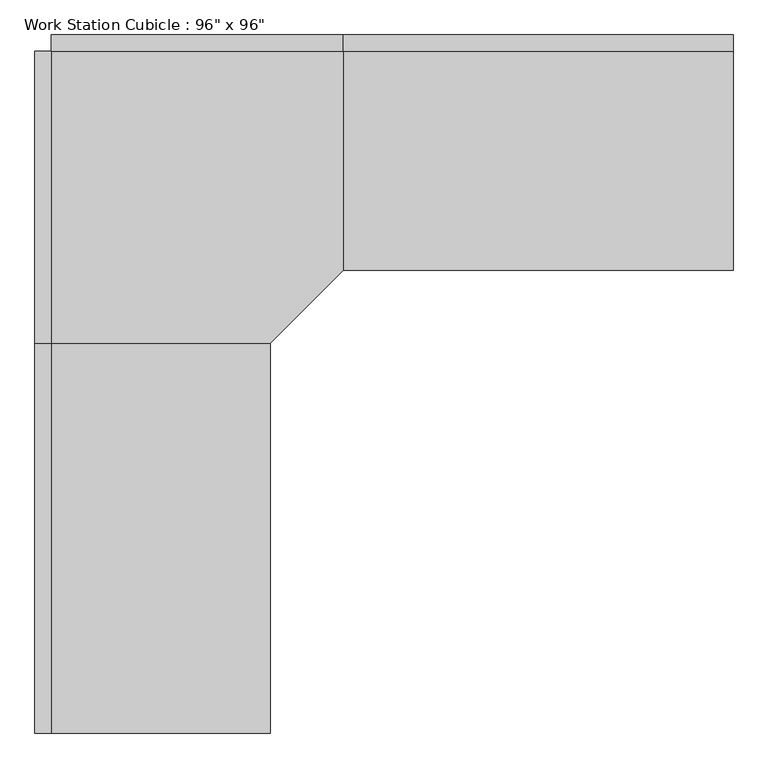
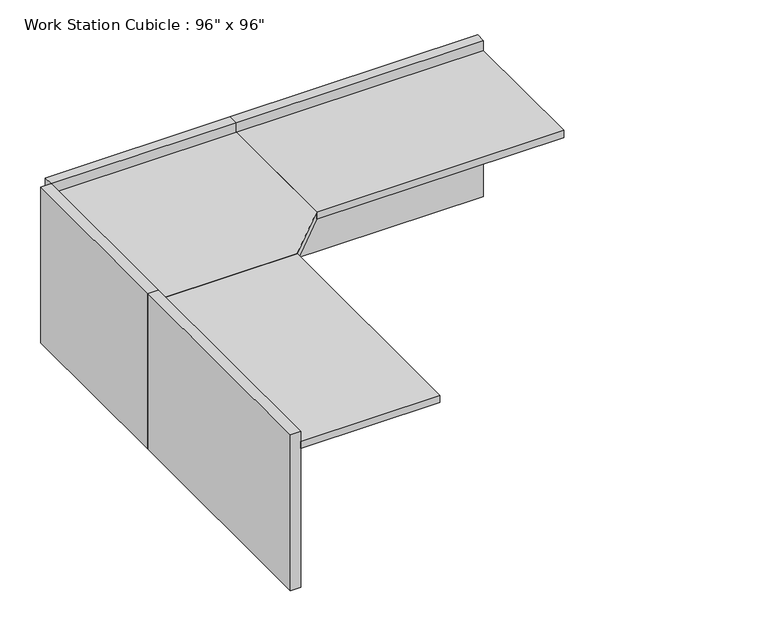
"""IFC4 building model written with IfcOpenShell, lengths in millimetres: furniture geometry."""

from ifc_helpers import new_model, si_unit, frame, origin, origin_with_axes, place, context, project, spatial, polyline, outline, extrude, source, transform, mapped, element, save


def furniture_4f0cce40(model_context):
    return source(origin(), model_context, "Body", "SweptSolid", [
        extrude(outline(polyline([(-80.9317522, -545.8230076), (833.4682478, -545.8230076), (833.4682478, -1231.6230076), (604.8682478, -1460.2230076), (-80.9317522, -1460.2230076), (-80.9317522, -545.8230076)])), frame((0.0, 0.0, 723.9), z_axis=(0.0, 0.0, 1.0), x_axis=(1.0, 0.0, 0.0)), (0.0, 0.0, 1.0), 38.1),
        extrude(outline(polyline([(604.8682478, -2679.4230076), (-80.9317522, -2679.4230076), (-80.9317522, -1460.2230076), (604.8682478, -1460.2230076), (604.8682478, -2679.4230076)])), frame((0.0, 0.0, 723.9), z_axis=(0.0, 0.0, 1.0), x_axis=(1.0, 0.0, 0.0)), (0.0, 0.0, 1.0), 38.1),
        extrude(outline(polyline([(2052.6682478, -1231.6230076), (833.4682478, -1231.6230076), (833.4682478, -545.8230076), (2052.6682478, -545.8230076), (2052.6682478, -1231.6230076)])), frame((0.0, 0.0, 723.9), z_axis=(0.0, 0.0, 1.0), x_axis=(1.0, 0.0, 0.0)), (0.0, 0.0, 1.0), 38.1),
        extrude(outline(polyline([(2052.6682478, -545.8230076), (833.4682478, -545.8230076), (833.4682478, -495.0230076), (2052.6682478, -495.0230076), (2052.6682478, -545.8230076)])), origin_with_axes(), (0.0, 0.0, 1.0), 812.8),
        extrude(outline(polyline([(833.4682478, -545.8230076), (-80.9317522, -545.8230076), (-80.9317522, -495.0230076), (833.4682478, -495.0230076), (833.4682478, -545.8230076)])), origin_with_axes(), (0.0, 0.0, 1.0), 812.8),
        extrude(outline(polyline([(-80.9317522, -1460.2230076), (-131.7317522, -1460.2230076), (-131.7317522, -545.8230076), (-80.9317522, -545.8230076), (-80.9317522, -1460.2230076)])), origin_with_axes(), (0.0, 0.0, 1.0), 812.8),
        extrude(outline(polyline([(-80.9317522, -2679.4230076), (-131.7317522, -2679.4230076), (-131.7317522, -1460.2230076), (-80.9317522, -1460.2230076), (-80.9317522, -2679.4230076)])), origin_with_axes(), (0.0, 0.0, 1.0), 812.8),
    ])


if __name__ == "__main__":
    model = new_model("IFC4")
    model_context = context("Model", 3, world=origin())
    ifc_project = project(units=[si_unit("LENGTHUNIT", "METRE", prefix="MILLI")], contexts=[model_context])
    site = spatial("IfcSite", under=ifc_project)
    building = spatial("IfcBuilding", under=site)
    placement = place(None, origin())
    furniture_shape = furniture_4f0cce40(model_context)
    element("IfcFurniture", 1, ObjectType="Work Station Cubicle : 96\" x 96\"", at=placement, inside=building, context=model_context, shape_type="MappedRepresentation", body=[
        mapped(furniture_shape, transform((0.0, 0.0, 0.0), x_axis=(1.0, 0.0, 0.0), y_axis=(0.0, 1.0, 0.0), z_axis=(0.0, 0.0, 1.0))),
    ])
    save(model, "model.ifc")

# Revit data of these elements
# Type "Work Station Cubicle : 96\" x 96\""
#   Assembly Code = "E2020"
#   Desktop Height = 2' - 6"
#   Desktop1 Width = 2' - 3"
#   Desktop2 Width = 2' - 3"
#   Panel Height = 2' - 8"
#   Panel1 Length = 4' - 0"
#   Panel2 Length = 4' - 0"
#   Cube Panel Material = Textile - Light Gray
#   Work Top Material = Laminate, Ivory, Matte
#   Default Elevation = 0
# Element 1 (IfcFurniture, "Work Station Cubicle : 96\" x 96\"")
#   Materials on its faces: "Textile - Light Gray", "Laminate, Ivory, Matte"
# Materials
#   "Textile - Light Gray": class "Fabric", colour RGB 204 204 204, transparency 0
#   "Laminate, Ivory, Matte": class "Plastic", colour RGB 247 247 239, transparency 0, Description = "Plastic Laminate - Ivory, Matte", Cost = 0
